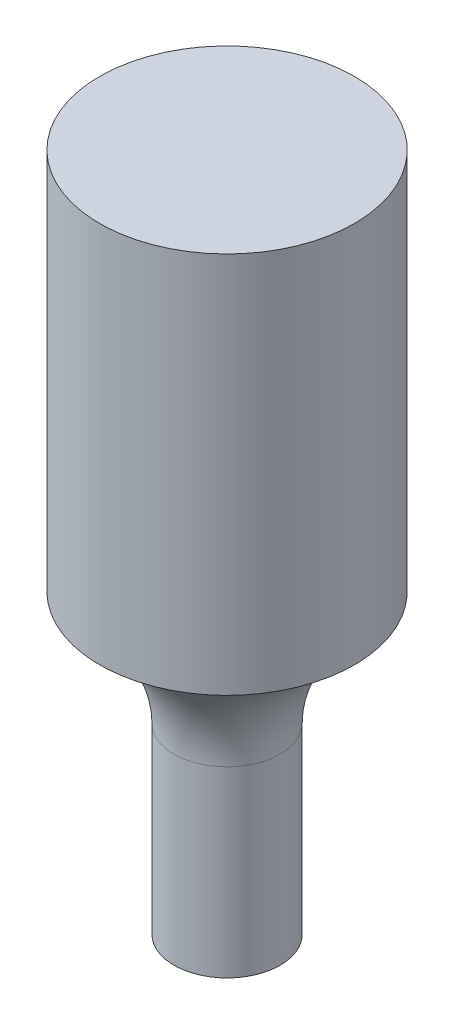
SolidWorks part; units mm, degrees
material "Plain Carbon Steel"
ref_plane "Front Plane" through (0, 0, 0) normal (0, 0, 1) x (1, 0, 0)
ref_plane "Top Plane" through (0, 0, 0) normal (0, 1, 0) x (1, 0, 0)
ref_plane "Right Plane" through (0, 0, 0) normal (1, 0, 0) x (0, 0, -1)
sketch "Punch Profile Sketch" plane through (0, 0, 0) normal (0, 0, 1) x (1, 0, 0)
  line L0 (0, 0) -> (0, 32) construction
  line L1 (0, 0) -> (-2.5, 0)
  line L2 (0, 32) -> (-6, 32)
  line L3 (-6, 32) -> (-6, 14)
  line L4 (-2.5, 0) -> (-2.5, 8.6102)
  line L5 (0, 0) -> (0, 32)
  arc A0 (-6, 14) -> (-2.5, 8.6102) centre (-8.4, 8.6102) cw
  dimension "D5" = 5.9
  dimension "D1" = 14
  dimension "D2" = 2.5
  dimension "D3" = 6
  dimension "D4" = 18
revolve "Punch Body Revolve" add sketch "Punch Profile Sketch" angle 360 about L0
